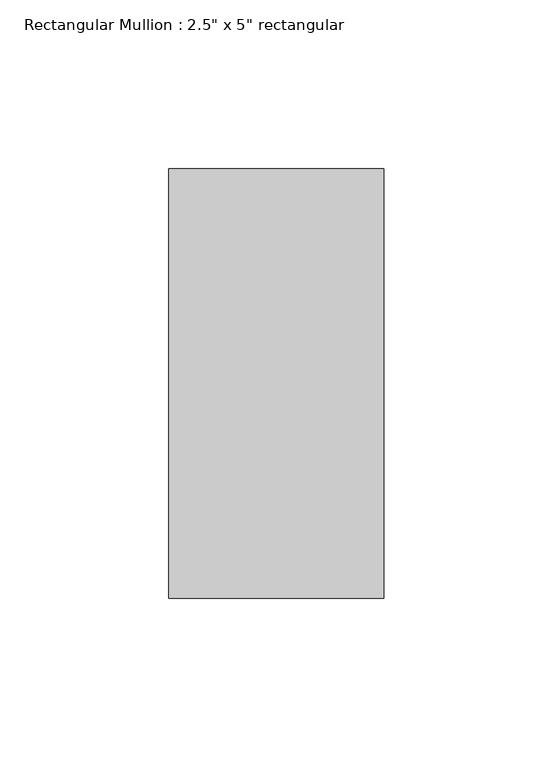
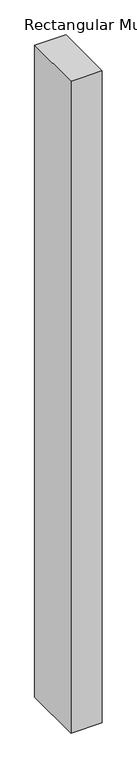
"""IFC4 building model written with IfcOpenShell, lengths in millimetres: member geometry."""

from ifc_helpers import new_model, si_unit, frame, origin, place, context, project, spatial, polyline, outline, extrude, source, transform, mapped, element, save


def member_f07b7441(model_context):
    return source(origin(), model_context, "Body", "SweptSolid", [
        extrude(outline(polyline([(0.0, 63.5), (0.0, -63.5), (-63.5, -63.5), (-63.5, 63.5), (0.0, 63.5)])), frame((0.0, 0.0, -1397.0), z_axis=(0.0, 0.0, 1.0), x_axis=(1.0, 0.0, 0.0)), (0.0, 0.0, 1.0), 1397.0),
    ])


if __name__ == "__main__":
    model = new_model("IFC4")
    model_context = context("Model", 3, world=origin())
    ifc_project = project(units=[si_unit("LENGTHUNIT", "METRE", prefix="MILLI")], contexts=[model_context])
    site = spatial("IfcSite", under=ifc_project)
    building = spatial("IfcBuilding", under=site)
    placement = place(None, origin())
    member_shape = member_f07b7441(model_context)
    element("IfcMember", 1, ObjectType="Rectangular Mullion : 2.5\" x 5\" rectangular", at=placement, inside=building, context=model_context, shape_type="MappedRepresentation", body=[
        mapped(member_shape, transform((0.0, 0.0, 0.0), x_axis=(1.0, 0.0, 0.0), y_axis=(0.0, 1.0, 0.0), z_axis=(0.0, 0.0, 1.0))),
    ])
    save(model, "model.ifc")

# Revit data of these elements
# Type "Rectangular Mullion : 2.5\" x 5\" rectangular"
#   built-in parameter 1007304 = 0.416667 (stored number, unit not read)
#   built-in parameter 1007301 = 0.104167 (stored number, unit not read)
#   built-in parameter 1007300 = 0.104167 (stored number, unit not read)
# Element 1 (IfcMember, "Rectangular Mullion : 2.5\" x 5\" rectangular")
#   Materials on its faces: "Aluminum"
# Materials
#   "Aluminum": class "Metal", colour RGB 247 247 247, transparency 0, Description = "Aluminum 6061", Cost = 0
